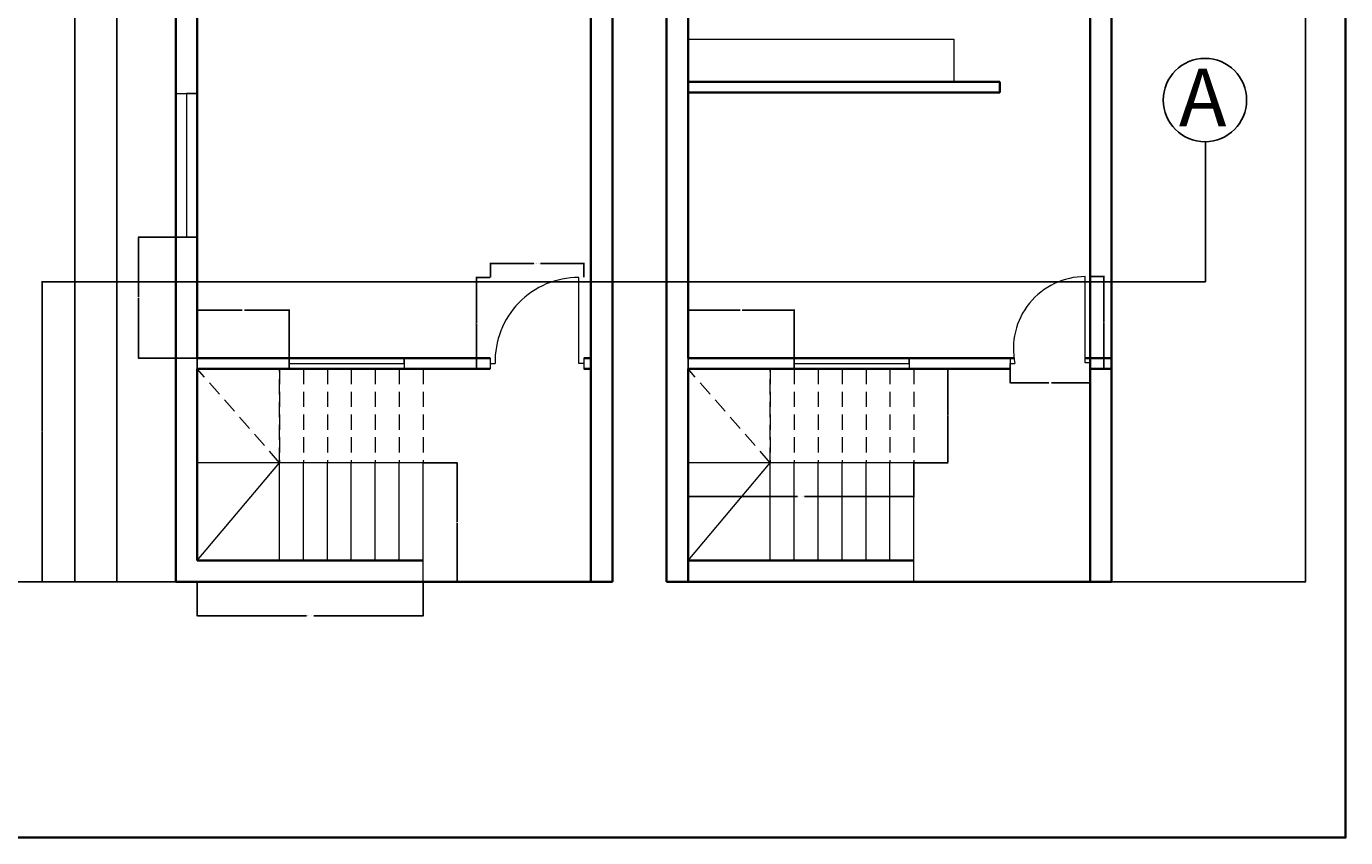
# Model space of a CAD drawing. Units: inches. Extents: x 2169 to 3181, y 1824 to 2912.
# Tile 3 of 5: x 2630 to 3181, y 1824 to 2163. Entities that reach past the tile are written whole.
import ezdxf

# ---------------------------------------------------------------- set-up
doc = ezdxf.new("R2010")
doc.units = ezdxf.units.IN
doc.linetypes.add('DASHED2', pattern=[9.525, 6.35, -3.175])
for name, color, linetype, lineweight in [('A-ANNO-DIMS', 2, 'Continuous', 18), ('A-ANNO-SYMB', 7, 'Continuous', 25), ('A-ANNO-TTLB', 7, 'Continuous', 35), ('A-DOOR', 3, 'Continuous', 18), ('A-FLOR-CASE', 8, 'Continuous', 18), ('A-FLOR-STRS', 7, 'Continuous', 18), ('A-FLOR-STRS-OVHD', 253, 'DASHED2', 13), ('A-GLAZ', 4, 'Continuous', 18), ('A-WALL', 7, 'Continuous', 35)]:
    doc.layers.add(name, color=color, linetype=linetype, lineweight=lineweight)
doc.styles.get("Standard").update_dxf_attribs({"font": 'arial.ttf'})
doc.dimstyles.get("Standard").update_dxf_attribs({"dimtxt": 0.18, "dimasz": 0.18, "dimexe": 0.18, "dimexo": 0.0625, "dimgap": 0.09, "dimtad": 0, "dimtih": 1, "dimtoh": 1, "dimdec": 4, "dimzin": 0, "dimdsep": 46, "dimtxsty": 'Standard', "dimcen": 0.09, "dimadec": 0, "dimazin": 0, "dimtfac": 1, "dimtdec": 4, "dimtofl": 0, "dimtmove": 0, "dimatfit": 3, "dimfxl": 1, "dimtolj": 1, "dimtzin": 0, "dimarcsym": 0})

# ---------------------------------------------------------------- blocks, each defined once
blk = doc.blocks.new('DOOR-ENTRY-G-36IN')
for p, q in [((0, 0), (0, 36)), ((-37.01, 2.25), (-37.01, -2.25)), ((2, 2.25), (2, -2.25)), ((-37.01, 0), (-35.01, 0)), ((2, 0), (0, 0))]:
    blk.add_line(p, q)
blk.add_arc((0, 0.98), 35.02, 90, 181.6016)
blk = doc.blocks.new('DOOR-ENTRY-U-36IN')
for p, q in [((0, 0), (0, 36)), ((-31.41, 1.93), (-31.41, 1.93)), ((-31.41, 1.93), (-31.41, -2.57)), ((2, 0), (0, 0)), ((-31.41, -2.57), (-31.41, -0.32)), ((-31.41, -0.32), (-31.41, -0.32)), ((-31.41, -0.32), (-29.41, -0.32))]:
    blk.add_line(p, q)
blk.add_arc((0, 5.93), 30.07, 90, 192.0072)
blk = doc.blocks.new('WIN-60IN')
for p, q in [((4.5, 60), (0, 60)), ((0, 60), (9, 60)), ((4.5, 0), (4.5, 60)), ((0, 0), (9, 0)), ((9, 0), (4.5, 0)), ((9, 0), (9, 0))]:
    blk.add_line(p, q)
blk = doc.blocks.new('WIN-48IN')
for p, q in [((0, 0), (0, 4.5)), ((0, 4.5), (0, 2.25)), ((0, 2.25), (48, 2.25)), ((48, 2.25), (48, 4.5)), ((48, 4.5), (48, 0))]:
    blk.add_line(p, q)
blk = doc.blocks.new('STAIR-RETURN-LOWER')
for p, q in [((94.36, 49.81), (0, 49.81)), ((0, 9), (34.36, 49.81)), ((34.36, 9), (34.36, 49.81)), ((44.36, 9), (44.36, 49.81)), ((54.36, 9), (54.36, 49.81)), ((64.36, 9), (64.36, 49.81)), ((74.36, 9), (74.36, 49.81)), ((84.36, 9), (84.36, 49.81)), ((94.36, 0), (94.36, 49.81))]:
    blk.add_line(p, q)
blk = doc.blocks.new('STAIR-RETURN-UPPER')
for p, q in [((34.36, 0), (0, 39.19)), ((34.36, 0), (34.36, 39.19)), ((34.36, 39.19), (34.36, 0)), ((44.36, 39.19), (44.36, 0)), ((54.36, 39.19), (54.36, 0)), ((64.36, 39.19), (64.36, 0)), ((74.36, 39.19), (74.36, 0)), ((84.36, 39.19), (84.36, 0)), ((94.36, 39.19), (94.36, 0))]:
    blk.add_line(p, q)
blk = doc.blocks.new('*D27')
at = {"layer": 'A-ANNO-DIMS', "color": 0, "lineweight": -2, "transparency": 16777216}
for p, q in [((2700.96, 1930.33), (2700.96, 1916.06)), ((2795.32, 1930.33), (2795.32, 1916.06)), ((2701.14, 1916.24), (2746.64, 1916.24)), ((2795.14, 1916.24), (2749.64, 1916.24))]:
    blk.add_line(p, q, dxfattribs=at)
at = {"layer": 'A-ANNO-DIMS', "color": 0, "transparency": 16777216}
for points in [[(2701.14, 1916.27), (2701.14, 1916.21), (2700.96, 1916.24)], [(2795.14, 1916.27), (2795.14, 1916.21), (2795.32, 1916.24)]]:
    blk.add_solid(points, dxfattribs=at)
at = {"layer": 'Defpoints', "color": 0, "transparency": 16777216}
for p in [(2700.96, 1930.39), (2795.32, 1930.39), (2795.32, 1916.24)]:
    blk.add_point(p, dxfattribs=at)
at = {"layer": 'A-ANNO-DIMS', "color": 0, "transparency": 16777216, "insert": (2748.14, 1916.24), "char_height": 0.18, "attachment_point": 5}
blk.add_mtext('\\A1;LOWER FLIGHT 94 TYP.', dxfattribs=at)
blk = doc.blocks.new('*D28')
at = {"layer": 'A-ANNO-DIMS', "color": 0, "lineweight": -2, "transparency": 16777216}
for p, q in [((2795.38, 1980.2), (2809.66, 1980.2)), ((2809.48, 1980.02), (2809.48, 1955.48)), ((2809.48, 1930.57), (2809.48, 1955.12)), ((2795.38, 1930.39), (2809.66, 1930.39))]:
    blk.add_line(p, q, dxfattribs=at)
at = {"layer": 'A-ANNO-DIMS', "color": 0, "transparency": 16777216}
for points in [[(2809.45, 1980.02), (2809.51, 1980.02), (2809.48, 1980.2)], [(2809.45, 1930.57), (2809.51, 1930.57), (2809.48, 1930.39)]]:
    blk.add_solid(points, dxfattribs=at)
at = {"layer": 'Defpoints', "color": 0, "transparency": 16777216}
for p in [(2795.32, 1980.2), (2809.48, 1980.2), (2795.32, 1930.39)]:
    blk.add_point(p, dxfattribs=at)
at = {"layer": 'A-ANNO-DIMS', "color": 0, "transparency": 16777216, "insert": (2809.48, 1955.3), "char_height": 0.18, "attachment_point": 5}
blk.add_mtext('\\A1;50 TYP.', dxfattribs=at)
blk = doc.blocks.new('*D29')
at = {"layer": 'A-ANNO-DIMS', "color": 0, "lineweight": -2, "transparency": 16777216}
for p, q in [((2906.05, 1980.14), (2906.05, 1965.87)), ((3000.42, 1980.14), (3000.42, 1965.87)), ((2906.23, 1966.05), (2951.76, 1966.05)), ((3000.24, 1966.05), (2954.71, 1966.05))]:
    blk.add_line(p, q, dxfattribs=at)
at = {"layer": 'A-ANNO-DIMS', "color": 0, "transparency": 16777216}
for points in [[(2906.23, 1966.08), (2906.23, 1966.02), (2906.05, 1966.05)], [(3000.24, 1966.08), (3000.24, 1966.02), (3000.42, 1966.05)]]:
    blk.add_solid(points, dxfattribs=at)
at = {"layer": 'Defpoints', "color": 0, "transparency": 16777216}
for p in [(2906.05, 1980.2), (3000.42, 1980.2), (3000.42, 1966.05)]:
    blk.add_point(p, dxfattribs=at)
at = {"layer": 'A-ANNO-DIMS', "color": 0, "transparency": 16777216, "insert": (2953.24, 1966.05), "char_height": 0.18, "attachment_point": 5}
blk.add_mtext('\\A1;UPPER FLIGHT 94 TYP.', dxfattribs=at)
blk = doc.blocks.new('*D30')
at = {"layer": 'A-ANNO-DIMS', "color": 0, "lineweight": -2, "transparency": 16777216}
for p, q in [((3000.48, 2019.39), (3014.75, 2019.39)), ((3014.57, 2019.21), (3014.57, 1999.98)), ((3014.57, 1980.38), (3014.57, 1999.62)), ((3000.48, 1980.2), (3014.75, 1980.2))]:
    blk.add_line(p, q, dxfattribs=at)
at = {"layer": 'A-ANNO-DIMS', "color": 0, "transparency": 16777216}
for points in [[(3014.54, 2019.21), (3014.6, 2019.21), (3014.57, 2019.39)], [(3014.54, 1980.38), (3014.6, 1980.38), (3014.57, 1980.2)]]:
    blk.add_solid(points, dxfattribs=at)
at = {"layer": 'Defpoints', "color": 0, "transparency": 16777216}
for p in [(3000.42, 2019.39), (3014.57, 2019.39), (3000.42, 1980.2)]:
    blk.add_point(p, dxfattribs=at)
at = {"layer": 'A-ANNO-DIMS', "color": 0, "transparency": 16777216, "insert": (3014.57, 1999.8), "char_height": 0.18, "attachment_point": 5}
blk.add_mtext('\\A1;39 TYP.', dxfattribs=at)
blk = doc.blocks.new('*D35')
at = {"layer": 'A-ANNO-DIMS', "color": 0, "lineweight": -2, "transparency": 16777216}
for p, q in [((2823.41, 2057.7), (2823.41, 2063.67)), ((2823.59, 2063.49), (2841.52, 2063.49)), ((2862.24, 2063.49), (2844.31, 2063.49)), ((2862.42, 2057.7), (2862.42, 2063.67))]:
    blk.add_line(p, q, dxfattribs=at)
at = {"layer": 'A-ANNO-DIMS', "color": 0, "transparency": 16777216}
for points in [[(2823.59, 2063.52), (2823.59, 2063.46), (2823.41, 2063.49)], [(2862.24, 2063.52), (2862.24, 2063.46), (2862.42, 2063.49)]]:
    blk.add_solid(points, dxfattribs=at)
at = {"layer": 'Defpoints', "color": 0, "transparency": 16777216}
for p in [(2862.42, 2063.49), (2823.41, 2057.64), (2862.42, 2057.64)]:
    blk.add_point(p, dxfattribs=at)
at = {"layer": 'A-ANNO-DIMS', "color": 0, "transparency": 16777216, "insert": (2842.91, 2063.49), "char_height": 0.18, "attachment_point": 5}
blk.add_mtext('\\A1;ENTRY DOOR 39 TYP.', dxfattribs=at)
blk = doc.blocks.new('*D36')
at = {"layer": 'A-ANNO-DIMS', "color": 0, "lineweight": -2, "transparency": 16777216}
for p, q in [((2823.35, 2057.64), (2817.38, 2057.64)), ((2817.56, 2057.46), (2817.56, 2038.7)), ((2817.56, 2019.57), (2817.56, 2038.34)), ((2823.35, 2019.39), (2817.38, 2019.39))]:
    blk.add_line(p, q, dxfattribs=at)
at = {"layer": 'A-ANNO-DIMS', "color": 0, "transparency": 16777216}
for points in [[(2817.53, 2057.46), (2817.59, 2057.46), (2817.56, 2057.64)], [(2817.53, 2019.57), (2817.59, 2019.57), (2817.56, 2019.39)]]:
    blk.add_solid(points, dxfattribs=at)
at = {"layer": 'Defpoints', "color": 0, "transparency": 16777216}
for p in [(2817.56, 2057.64), (2823.41, 2057.64), (2823.41, 2019.39)]:
    blk.add_point(p, dxfattribs=at)
at = {"layer": 'A-ANNO-DIMS', "color": 0, "transparency": 16777216, "insert": (2817.56, 2038.52), "char_height": 0.18, "attachment_point": 5}
blk.add_mtext('\\A1;38 TYP.', dxfattribs=at)
blk = doc.blocks.new('*D41')
at = {"layer": 'A-ANNO-DIMS', "color": 0, "lineweight": -2, "transparency": 16777216}
for p, q in [((3074.12, 2057.96), (3080.02, 2057.96)), ((3079.84, 2057.78), (3079.84, 2038.86)), ((3079.84, 2019.57), (3079.84, 2038.49)), ((3074.12, 2019.39), (3080.02, 2019.39))]:
    blk.add_line(p, q, dxfattribs=at)
at = {"layer": 'A-ANNO-DIMS', "color": 0, "transparency": 16777216}
for points in [[(3079.81, 2057.78), (3079.87, 2057.78), (3079.84, 2057.96)], [(3079.81, 2019.57), (3079.87, 2019.57), (3079.84, 2019.39)]]:
    blk.add_solid(points, dxfattribs=at)
at = {"layer": 'Defpoints', "color": 0, "transparency": 16777216}
for p in [(3074.05, 2057.96), (3079.84, 2057.96), (3074.05, 2019.39)]:
    blk.add_point(p, dxfattribs=at)
at = {"layer": 'A-ANNO-DIMS', "color": 0, "transparency": 16777216, "insert": (3079.84, 2038.68), "char_height": 0.18, "attachment_point": 5}
blk.add_mtext('\\A1;ENTRY DOOR 39 TYP.', dxfattribs=at)
blk = doc.blocks.new('*D42')
at = {"layer": 'A-ANNO-DIMS', "color": 0, "lineweight": -2, "transparency": 16777216}
for p, q in [((3040.64, 2019.33), (3040.64, 2013.43)), ((3074.05, 2019.33), (3074.05, 2013.43)), ((3040.82, 2013.61), (3056.82, 2013.61)), ((3073.87, 2013.61), (3057.88, 2013.61))]:
    blk.add_line(p, q, dxfattribs=at)
at = {"layer": 'A-ANNO-DIMS', "color": 0, "transparency": 16777216}
for points in [[(3040.82, 2013.64), (3040.82, 2013.58), (3040.64, 2013.61)], [(3073.87, 2013.64), (3073.87, 2013.58), (3074.05, 2013.61)]]:
    blk.add_solid(points, dxfattribs=at)
at = {"layer": 'Defpoints', "color": 0, "transparency": 16777216}
for p in [(3040.64, 2019.39), (3074.05, 2019.39), (3074.05, 2013.61)]:
    blk.add_point(p, dxfattribs=at)
at = {"layer": 'A-ANNO-DIMS', "color": 0, "transparency": 16777216, "insert": (3057.35, 2013.61), "char_height": 0.18, "attachment_point": 5}
blk.add_mtext('\\A1;33 TYP.', dxfattribs=at)
blk = doc.blocks.new('*D56')
at = {"layer": 'A-ANNO-DIMS', "color": 0, "lineweight": -2, "transparency": 16777216}
for p, q in [((2623.43, 2417.39), (2649.9, 2417.39)), ((2649.72, 2417.21), (2649.72, 2174.07)), ((2649.72, 1930.57), (2649.72, 2173.71)), ((2623.43, 1930.39), (2649.9, 1930.39))]:
    blk.add_line(p, q, dxfattribs=at)
at = {"layer": 'A-ANNO-DIMS', "color": 0, "transparency": 16777216}
for points in [[(2649.69, 2417.21), (2649.75, 2417.21), (2649.72, 2417.39)], [(2649.69, 1930.57), (2649.75, 1930.57), (2649.72, 1930.39)]]:
    blk.add_solid(points, dxfattribs=at)
at = {"layer": 'Defpoints', "color": 0, "transparency": 16777216}
for p in [(2623.37, 2417.39), (2649.72, 2417.39), (2623.37, 1930.39)]:
    blk.add_point(p, dxfattribs=at)
at = {"layer": 'A-ANNO-DIMS', "color": 0, "transparency": 16777216, "insert": (2649.72, 2173.89), "char_height": 0.18, "attachment_point": 5}
blk.add_mtext('\\A1;487', dxfattribs=at)
blk = doc.blocks.new('*D59')
at = {"layer": 'A-ANNO-DIMS', "color": 0, "lineweight": -2, "transparency": 16777216}
for p, q in [((2700.96, 2019.45), (2700.96, 2044.17)), ((2701.14, 2043.99), (2719.71, 2043.99)), ((2739.2, 2043.99), (2720.63, 2043.99)), ((2739.38, 2019.45), (2739.38, 2044.17))]:
    blk.add_line(p, q, dxfattribs=at)
at = {"layer": 'A-ANNO-DIMS', "color": 0, "transparency": 16777216}
for points in [[(2701.14, 2044.02), (2701.14, 2043.96), (2700.96, 2043.99)], [(2739.2, 2044.02), (2739.2, 2043.96), (2739.38, 2043.99)]]:
    blk.add_solid(points, dxfattribs=at)
at = {"layer": 'Defpoints', "color": 0, "transparency": 16777216}
for p in [(2739.38, 2043.99), (2700.96, 2019.39), (2739.38, 2019.39)]:
    blk.add_point(p, dxfattribs=at)
at = {"layer": 'A-ANNO-DIMS', "color": 0, "transparency": 16777216, "insert": (2720.17, 2043.99), "char_height": 0.18, "attachment_point": 5}
blk.add_mtext('\\A1;38.426', dxfattribs=at)
blk = doc.blocks.new('*D60')
at = {"layer": 'A-ANNO-DIMS', "color": 0, "lineweight": -2, "transparency": 16777216}
for p, q in [((2906.05, 2019.45), (2906.05, 2044.17)), ((2906.23, 2043.99), (2927.84, 2043.99)), ((2950.24, 2043.99), (2928.63, 2043.99)), ((2950.42, 2019.45), (2950.42, 2044.17))]:
    blk.add_line(p, q, dxfattribs=at)
at = {"layer": 'A-ANNO-DIMS', "color": 0, "transparency": 16777216}
for points in [[(2906.23, 2044.02), (2906.23, 2043.96), (2906.05, 2043.99)], [(2950.24, 2044.02), (2950.24, 2043.96), (2950.42, 2043.99)]]:
    blk.add_solid(points, dxfattribs=at)
at = {"layer": 'Defpoints', "color": 0, "transparency": 16777216}
for p in [(2950.42, 2043.99), (2906.05, 2019.39), (2950.42, 2019.39)]:
    blk.add_point(p, dxfattribs=at)
at = {"layer": 'A-ANNO-DIMS', "color": 0, "transparency": 16777216, "insert": (2928.24, 2043.99), "char_height": 0.18, "attachment_point": 5}
blk.add_mtext('\\A1;44.36', dxfattribs=at)
blk = doc.blocks.new('*D61')
at = {"layer": 'A-ANNO-DIMS', "color": 0, "lineweight": -2, "transparency": 16777216}
for p, q in [((2700.89, 2074.51), (2676.18, 2074.51)), ((2676.36, 2074.33), (2676.36, 2049.39)), ((2676.36, 2024.07), (2676.36, 2049.02)), ((2700.89, 2023.89), (2676.18, 2023.89))]:
    blk.add_line(p, q, dxfattribs=at)
at = {"layer": 'A-ANNO-DIMS', "color": 0, "transparency": 16777216}
for points in [[(2676.33, 2074.33), (2676.39, 2074.33), (2676.36, 2074.51)], [(2676.33, 2024.07), (2676.39, 2024.07), (2676.36, 2023.89)]]:
    blk.add_solid(points, dxfattribs=at)
at = {"layer": 'Defpoints', "color": 0, "transparency": 16777216}
for p in [(2676.36, 2074.51), (2700.96, 2074.51), (2700.96, 2023.89)]:
    blk.add_point(p, dxfattribs=at)
at = {"layer": 'A-ANNO-DIMS', "color": 0, "transparency": 16777216, "insert": (2676.36, 2049.2), "char_height": 0.18, "attachment_point": 5}
blk.add_mtext('\\A1;50.62', dxfattribs=at)
blk = doc.blocks.new('*D65')
at = {"layer": 'A-ANNO-DIMS', "color": 0, "lineweight": -2, "transparency": 16777216}
for p, q in [((2691.89, 2417.39), (2667.18, 2417.39)), ((2667.36, 2417.21), (2667.36, 2174.07)), ((2667.36, 1930.57), (2667.36, 2173.71)), ((2691.89, 1930.39), (2667.18, 1930.39))]:
    blk.add_line(p, q, dxfattribs=at)
at = {"layer": 'A-ANNO-DIMS', "color": 0, "transparency": 16777216}
for points in [[(2667.33, 2417.21), (2667.39, 2417.21), (2667.36, 2417.39)], [(2667.33, 1930.57), (2667.39, 1930.57), (2667.36, 1930.39)]]:
    blk.add_solid(points, dxfattribs=at)
at = {"layer": 'Defpoints', "color": 0, "transparency": 16777216}
for p in [(2667.36, 2417.39), (2691.96, 2417.39), (2691.96, 1930.39)]:
    blk.add_point(p, dxfattribs=at)
at = {"layer": 'A-ANNO-DIMS', "color": 0, "transparency": 16777216, "insert": (2667.36, 2173.89), "char_height": 0.18, "attachment_point": 5}
blk.add_mtext('\\A1;487', dxfattribs=at)
blk = doc.blocks.new('*D67')
at = {"layer": 'A-ANNO-DIMS', "color": 0, "lineweight": -2, "transparency": 16777216}
for p, q in [((3083.12, 2417.39), (3164.24, 2417.39)), ((3164.06, 2417.21), (3164.06, 2174.07)), ((3164.06, 1930.57), (3164.06, 2173.71)), ((3083.12, 1930.39), (3164.24, 1930.39))]:
    blk.add_line(p, q, dxfattribs=at)
at = {"layer": 'A-ANNO-DIMS', "color": 0, "transparency": 16777216}
for points in [[(3164.03, 2417.21), (3164.09, 2417.21), (3164.06, 2417.39)], [(3164.03, 1930.57), (3164.09, 1930.57), (3164.06, 1930.39)]]:
    blk.add_solid(points, dxfattribs=at)
at = {"layer": 'Defpoints', "color": 0, "transparency": 16777216}
for p in [(3083.05, 2417.39), (3164.06, 2417.39), (3083.05, 1930.39)]:
    blk.add_point(p, dxfattribs=at)
at = {"layer": 'A-ANNO-DIMS', "color": 0, "transparency": 16777216, "insert": (3164.06, 2173.89), "char_height": 0.18, "attachment_point": 5}
blk.add_mtext('\\A1;487', dxfattribs=at)
blk = doc.blocks.new('*D68')
at = {"layer": 'A-ANNO-DIMS', "color": 0, "lineweight": -2, "transparency": 16777216}
for p, q in [((2660.6, 2055.76), (2635.88, 2055.76)), ((2636.06, 2055.58), (2636.06, 1993.26)), ((2636.06, 1930.57), (2636.06, 1992.9)), ((2691.89, 1930.39), (2635.88, 1930.39))]:
    blk.add_line(p, q, dxfattribs=at)
at = {"layer": 'A-ANNO-DIMS', "color": 0, "transparency": 16777216}
for points in [[(2636.03, 2055.58), (2636.09, 2055.58), (2636.06, 2055.76)], [(2636.03, 1930.57), (2636.09, 1930.57), (2636.06, 1930.39)]]:
    blk.add_solid(points, dxfattribs=at)
at = {"layer": 'Defpoints', "color": 0, "transparency": 16777216}
for p in [(2660.66, 2055.76), (2636.06, 1930.39), (2691.96, 1930.39)]:
    blk.add_point(p, dxfattribs=at)
at = {"layer": 'A-ANNO-DIMS', "color": 0, "transparency": 16777216, "insert": (2636.06, 1993.08), "char_height": 0.18, "attachment_point": 5}
blk.add_mtext('\\A1;125.37', dxfattribs=at)

msp = doc.modelspace()

# ---------------------------------------------------------------- linework, layer by layer
at = {"layer": 'A-ANNO-SYMB'}
for p, q in [((3122.331, 2055.7618), (3122.331, 2114.3171)), ((2660.6608, 2055.7618), (3122.331, 2055.7618))]:
    msp.add_line(p, q, dxfattribs=at)
msp.add_circle((3122.0397, 2131.7388), 17.4241, dxfattribs=at)
at = {"layer": 'A-ANNO-TTLB'}
msp.add_lwpolyline([(2168.7598, 2912.462), (3180.8253, 2912.462), (3180.8253, 1823.5481), (2168.7598, 1823.5481)], close=True, dxfattribs=at)
at = {"layer": 'A-FLOR-CASE'}
for p, q in [((2906.0534, 2157.1645), (3017.1436, 2157.1645)), ((3017.1436, 2157.1645), (3017.1436, 2139.3924))]:
    msp.add_line(p, q, dxfattribs=at)
at = {"layer": 'A-FLOR-STRS'}
msp.add_line((2700.9572, 1939.3924), (2700.9572, 1939.3924), dxfattribs=at)
at = {"layer": 'A-GLAZ'}
msp.add_line((2950.4168, 2019.3924), (2950.4168, 2019.3924), dxfattribs=at)
at = {"layer": 'A-WALL'}
for p, q in [((2691.9572, 2417.3924), (2691.9572, 1930.3924)), ((2874.4572, 2417.3924), (2874.4572, 1930.3924)), ((2897.0534, 2417.3924), (2897.0534, 1930.3924)), ((3083.0534, 2417.3924), (3083.0534, 1930.3924)), ((2906.0534, 2408.3924), (2906.0534, 2023.8924)), ((3074.0534, 2408.3924), (3074.0534, 1930.3924)), ((2700.9572, 2319.8924), (2700.9572, 2023.8924)), ((2865.4572, 2263.8924), (2865.4572, 1930.3924)), ((2906.0534, 2139.3924), (3036.3523, 2139.3924)), ((3036.3523, 2139.3924), (3036.3523, 2139.3924)), ((3036.3523, 2139.3924), (3036.3523, 2134.8924)), ((2906.0534, 2134.8924), (3036.3523, 2134.8924)), ((2700.9572, 2023.8924), (2823.4085, 2023.8924)), ((2865.4572, 2023.8924), (2862.416, 2023.8924)), ((2906.0534, 2023.8924), (3042.2549, 2023.8924)), ((3072.0534, 2023.8924), (3083.0534, 2023.8924)), ((2700.9572, 2019.3924), (2823.4085, 2019.3924)), ((2700.9572, 2019.3924), (2700.9572, 1939.3924)), ((2862.416, 2019.3924), (2865.4572, 2019.3924)), ((2906.0534, 2019.3924), (2906.0534, 1930.3924)), ((2906.0534, 2019.3924), (3040.6448, 2019.3924)), ((3074.0534, 2019.3924), (3083.0534, 2019.3924)), ((2700.9572, 1939.3924), (2795.3206, 1939.3924)), ((2906.0534, 1939.3924), (3000.4168, 1939.3924)), ((2700.9572, 1930.3924), (2691.9572, 1930.3924)), ((2691.9572, 1930.3924), (2874.4572, 1930.3924)), ((2700.9572, 1930.3924), (2795.3206, 1930.3924)), ((2897.0534, 1930.3924), (3083.0534, 1930.3924)), ((3083.0534, 1930.3924), (3083.0534, 1930.3924))]:
    msp.add_line(p, q, dxfattribs=at)

# ---------------------------------------------------------------- block references
at = {"layer": 'A-DOOR'}
for name, p in [('DOOR-ENTRY-G-36IN', (2860.416, 2021.6424)), ('DOOR-ENTRY-U-36IN', (3072.0534, 2021.9638))]:
    msp.add_blockref(name, p, dxfattribs=at)
at = {"layer": 'A-FLOR-STRS'}
for p in [(2700.9576, 1930.392), (2906.0538, 1930.392), (2906.0538, 1930.392)]:
    msp.add_blockref('STAIR-RETURN-LOWER', p, dxfattribs=at)
at = {"layer": 'A-FLOR-STRS-OVHD'}
for p in [(2700.9576, 1980.202), (2906.0538, 1980.202), (2906.0538, 1980.202)]:
    msp.add_blockref('STAIR-RETURN-UPPER', p, dxfattribs=at)
at = {"layer": 'A-GLAZ', "extrusion": (0, 0, -1), "zscale": -1, "rotation": 180}
msp.add_blockref('WIN-60IN', (-2691.9576, 2134.5134), dxfattribs=at)
at = {"layer": 'A-GLAZ'}
for p in [(2739.3826, 2019.392), (2950.4166, 2019.392)]:
    msp.add_blockref('WIN-48IN', p, dxfattribs=at)

# ---------------------------------------------------------------- texts
at = {"layer": 'A-ANNO-SYMB', "insert": (3111.1359, 2144.8218), "char_height": 24, "attachment_point": 1}
msp.add_mtext('A', dxfattribs=at)

# ---------------------------------------------------------------- dimensions: what is measured, and where the dimension line sits
at = {"layer": 'A-ANNO-DIMS'}
for base, p1, p2, override, picture, middle in [((2649.7198, 2417.3924), (2623.3698, 1930.3924), (2623.3698, 2417.3924), {"dimdec": 0, "dimlfac": 1, "dimrnd": 0, "dimzin": 0, "dimdsep": 46, "dimlunit": 2}, '*D56', (2649.7198, 2173.8924)), ((2667.3572, 2417.3924), (2691.9572, 1930.3924), (2691.9572, 2417.3924), {"dimdec": 0, "dimlfac": 1, "dimrnd": 0, "dimzin": 0, "dimdsep": 46, "dimlunit": 2}, '*D65', (2667.3572, 2173.8924)), ((3164.0639, 2417.3924), (3083.0534, 1930.3924), (3083.0534, 2417.3924), {"dimdec": 0, "dimlfac": 1, "dimrnd": 0, "dimzin": 0, "dimdsep": 46, "dimlunit": 2}, '*D67', (3164.0639, 2173.8924)), ((2676.3572, 2074.5139), (2700.9572, 2023.8924), (2700.9572, 2074.5139), {"dimdec": 2, "dimlfac": 1, "dimrnd": 0, "dimzin": 0, "dimdsep": 46, "dimlunit": 2}, '*D61', (2676.3572, 2049.2032)), ((2636.0608, 1930.3924), (2660.6608, 2055.7618), (2691.9572, 1930.3924), {"dimdec": 2, "dimlfac": 1, "dimrnd": 0, "dimzin": 0, "dimdsep": 46, "dimlunit": 2}, '*D68', (2636.0608, 1993.0771))]:
    dim = msp.add_linear_dim(base=base, p1=p1, p2=p2, angle=90, dimstyle='Standard', override=override, dxfattribs=at)
    dim.commit()
    dim.dimension.update_dxf_attribs({"geometry": picture, "text_midpoint": middle})
for base, p1, p2, text, picture, middle in [((2862.416, 2063.4935), (2823.4085, 2057.6424), (2862.416, 2057.6424), 'ENTRY DOOR <> TYP.', '*D35', (2842.9122, 2063.4935)), ((3074.0534, 2013.6067), (3040.6448, 2019.3924), (3074.0534, 2019.3924), '<> TYP.', '*D42', (3057.3491, 2013.6067)), ((3000.4168, 1966.0471), (2906.0534, 1980.2016), (3000.4168, 1980.2016), 'UPPER FLIGHT <> TYP.', '*D29', (2953.2351, 1966.0471)), ((2795.3206, 1916.2379), (2700.9572, 1930.3924), (2795.3206, 1930.3924), 'LOWER FLIGHT <> TYP.', '*D27', (2748.1389, 1916.2379))]:
    dim = msp.add_linear_dim(base=base, p1=p1, p2=p2, text=text, dimstyle='Standard', override={"dimdec": 0, "dimlfac": 1, "dimrnd": 0, "dimzin": 0, "dimdsep": 46, "dimlunit": 2}, dxfattribs=at)
    dim.commit()
    dim.dimension.update_dxf_attribs({"geometry": picture, "text_midpoint": middle})
for base, p1, p2, text, picture, middle in [((2817.5573, 2057.6424), (2823.4085, 2019.3924), (2823.4085, 2057.6424), '<> TYP.', '*D36', (2817.5573, 2038.5174)), ((3079.8391, 2057.9638), (3074.0534, 2019.3924), (3074.0534, 2057.9638), 'ENTRY DOOR <> TYP.', '*D41', (3079.8391, 2038.6781)), ((3014.5713, 2019.3924), (3000.4168, 1980.2016), (3000.4168, 2019.3924), '<> TYP.', '*D30', (3014.5713, 1999.797)), ((2809.4751, 1980.2016), (2795.3206, 1930.3924), (2795.3206, 1980.2016), '<> TYP.', '*D28', (2809.4751, 1955.297))]:
    dim = msp.add_linear_dim(base=base, p1=p1, p2=p2, angle=90, text=text, dimstyle='Standard', override={"dimdec": 0, "dimlfac": 1, "dimrnd": 0, "dimzin": 0, "dimdsep": 46, "dimlunit": 2}, dxfattribs=at)
    dim.commit()
    dim.dimension.update_dxf_attribs({"geometry": picture, "text_midpoint": middle})
for base, p1, p2, override, picture, middle in [((2739.3828, 2043.9924), (2700.9572, 2019.3924), (2739.3828, 2019.3924), {"dimdec": 3, "dimlfac": 1, "dimrnd": 0, "dimzin": 0, "dimdsep": 46, "dimlunit": 2}, '*D59', (2720.17, 2043.9924)), ((2950.4168, 2043.9924), (2906.0534, 2019.3924), (2950.4168, 2019.3924), {"dimdec": 2, "dimlfac": 1, "dimrnd": 0, "dimzin": 0, "dimdsep": 46, "dimlunit": 2}, '*D60', (2928.2351, 2043.9924))]:
    dim = msp.add_linear_dim(base=base, p1=p1, p2=p2, dimstyle='Standard', override=override, dxfattribs=at)
    dim.commit()
    dim.dimension.update_dxf_attribs({"geometry": picture, "text_midpoint": middle})

doc.saveas('drawing.dxf')
